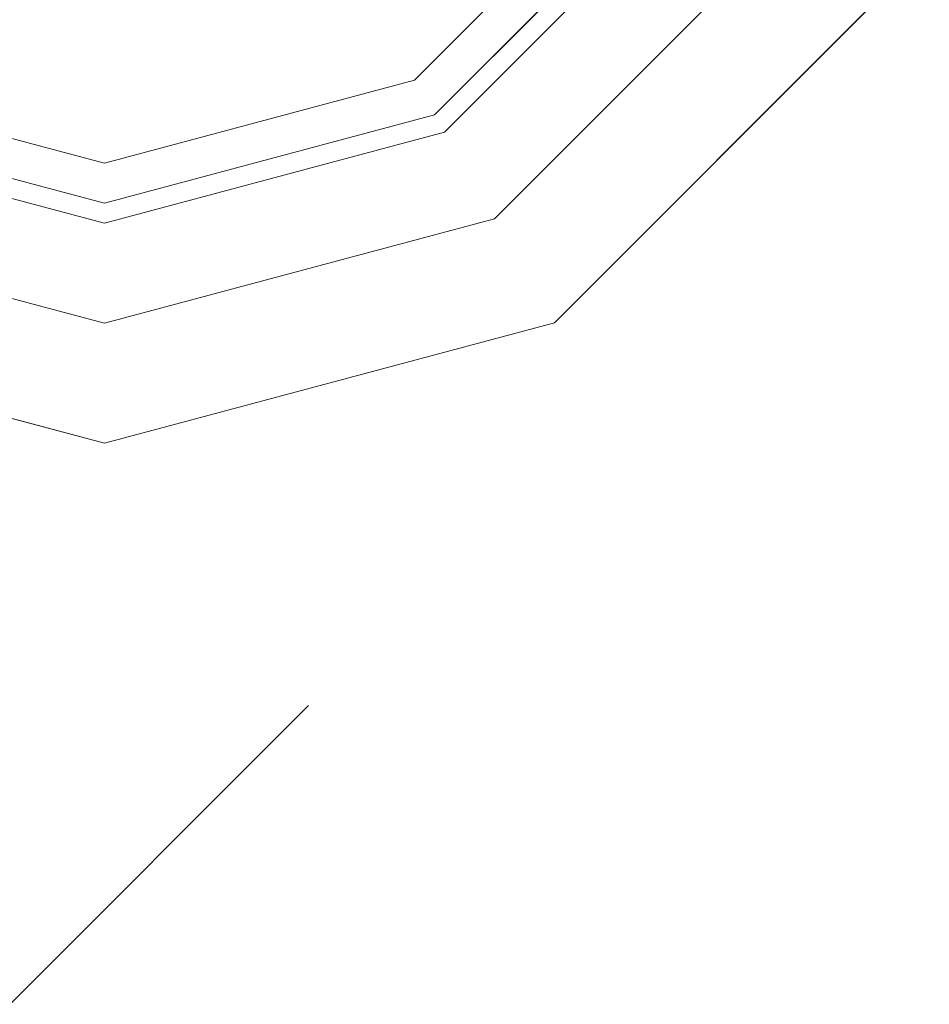
# Model space of a CAD drawing. Units: inches. Extents: x 375 to 1122, y 27 to 1069.
# Tile 134 of 155: x 725.559 to 731.16, y 900.211 to 906.27. Entities that reach past the tile are written whole.
import ezdxf

# ---------------------------------------------------------------- set-up
doc = ezdxf.new("R2010")
doc.units = ezdxf.units.IN
doc.layers.add('A-ANNO-DIMS', color=2, linetype='Continuous', lineweight=18)
doc.layers.add('Furniture', color=30, linetype='Continuous', lineweight=18)
doc.styles.get("Standard").update_dxf_attribs({"font": 'arial.ttf'})
doc.dimstyles.new('ISO-25', dxfattribs={"dimtxt": 12, "dimasz": 2.5, "dimexe": 1.5, "dimexo": 1.5, "dimtad": 1, "dimdec": 1, "dimlunit": 3, "dimtxsty": 'Standard', "dimblk": 'ARCHTICK', "dimcen": 2.5, "dimadec": 0, "dimazin": 0, "dimtfac": 1, "dimtdec": 1, "dimtmove": 0, "dimatfit": 3, "dimfxl": 1.5, "dimfxlon": 1, "dimarcsym": 0})

# ---------------------------------------------------------------- blocks, each defined once
blk = doc.blocks.new('A$C403C54AD')
blk.add_line((0.90685, 1.05977, -0.0006), (1.01943, 0.94723, -0.0006))
at = {"linetype": 'ByBlock'}
for points, invisible_edges in [([(0.81861, 1.08071, -0.03355), (0.84793, 1.09765, -0.02431), (0.79723, 1.14835, -0.02431), (0.7803, 1.11902, -0.03355)], 5), ([(0.84793, 1.09765, -0.0197), (0.83194, 1.08841, -0.0197), (0.78799, 1.13235, -0.0197), (0.79723, 1.14835, -0.0197)], 5), ([(0.83194, 1.08841, -0.0197), (0.81594, 1.07918, -0.02585), (0.77876, 1.11636, -0.02585), (0.78799, 1.13235, -0.0197)], 5), ([(0.81061, 1.0761, -0.04278), (0.81861, 1.08071, -0.03355), (0.7803, 1.11902, -0.03355), (0.77568, 1.11103, -0.04278)], 1), ([(0.81594, 1.07918, -0.02585), (0.72796, 1.02838, -0.02585), (0.72796, 1.02838, -0.02585), (0.77876, 1.11636, -0.02585)], 5), ([(0.83263, 1.02838, -0.03355), (0.86649, 1.02838, -0.02431), (0.84793, 1.09765, -0.02431), (0.81861, 1.08071, -0.03355)], 5), ([(0.86649, 1.02838, -0.0197), (0.84802, 1.02838, -0.0197), (0.83194, 1.08841, -0.0197), (0.84793, 1.09765, -0.0197)], 5), ([(0.84802, 1.02838, -0.0197), (0.82955, 1.02838, -0.02585), (0.81594, 1.07918, -0.02585), (0.83194, 1.08841, -0.0197)], 5), ([(0.82339, 1.02838, -0.04278), (0.83263, 1.02838, -0.03355), (0.81861, 1.08071, -0.03355), (0.81061, 1.0761, -0.04278)], 5), ([(0.82955, 1.02838, -0.02585), (0.72796, 1.02838, -0.02585), (0.72796, 1.02838, -0.02585), (0.81594, 1.07918, -0.02585)], 5), ([(0.81594, 0.97759, -0.02585), (0.72796, 1.02838, -0.02585), (0.72796, 1.02838, -0.02585), (0.82955, 1.02838, -0.02585)], 5), ([(0.77876, 0.94041, -0.02585), (0.72796, 1.02838, -0.02585), (0.72796, 1.02838, -0.02585), (0.81594, 0.97759, -0.02585)], 5), ([(0.81061, 0.98067, -0.04278), (0.81861, 0.97605, -0.03355), (0.83263, 1.02838, -0.03355), (0.82339, 1.02838, -0.04278)], 5), ([(0.83194, 0.96835, -0.0197), (0.81594, 0.97759, -0.02585), (0.82955, 1.02838, -0.02585), (0.84802, 1.02838, -0.0197)], 5), ([(0.81861, 0.97605, -0.03355), (0.84793, 0.95912, -0.02431), (0.86649, 1.02838, -0.02431), (0.83263, 1.02838, -0.03355)], 5), ([(0.84793, 0.95912, -0.0197), (0.83194, 0.96835, -0.0197), (0.84802, 1.02838, -0.0197), (0.86649, 1.02838, -0.0197)], 5)]:
    blk.add_3dface(points, dxfattribs=dict(at, invisible_edges=invisible_edges))
for points in [[(0.84793, 1.09765, -0.02431), (0.84793, 1.09765, -0.0197), (0.79723, 1.14835, -0.0197), (0.79723, 1.14835, -0.02431)], [(0.86649, 1.02838, -0.02431), (0.86649, 1.02838, -0.0197), (0.84793, 1.09765, -0.0197), (0.84793, 1.09765, -0.02431)], [(0.84793, 0.95912, -0.02431), (0.84793, 0.95912, -0.0197), (0.86649, 1.02838, -0.0197), (0.86649, 1.02838, -0.02431)]]:
    blk.add_3dface(points, dxfattribs=at)
blk = doc.blocks.new('_ArchTick')
at = {"color": 0, "linetype": 'ByBlock', "const_width": 0.15}
blk.add_lwpolyline([(-0.5, -0.5), (0.5, 0.5)], dxfattribs=at)
blk = doc.blocks.new('*D73')
at = {"layer": 'A-ANNO-DIMS', "color": 0, "lineweight": -2, "transparency": 16777216}
for p, q in [((686.7573, 932.4277), (686.7573, 929.4277)), ((770.7573, 932.4277), (770.7573, 929.4277)), ((686.7573, 930.9277), (770.7573, 930.9277)), ((770.7573, 930.9277), (987.6096, 930.9277))]:
    blk.add_line(p, q, dxfattribs=at)
at = {"layer": 'Defpoints', "color": 0, "transparency": 16777216}
for p in [(686.7573, 943.5277), (770.7573, 943.5277), (770.7573, 930.9277)]:
    blk.add_point(p, dxfattribs=at)
at = {"layer": 'A-ANNO-DIMS', "color": 0, "lineweight": -2, "transparency": 16777216, "xscale": 2.5, "yscale": 2.5, "zscale": 2.5, "rotation": 180}
blk.add_blockref('_ArchTick', (686.7573, 930.9277), dxfattribs=at)
at = {"layer": 'A-ANNO-DIMS', "color": 0, "lineweight": -2, "transparency": 16777216, "xscale": 2.5, "yscale": 2.5, "zscale": 2.5}
blk.add_blockref('_ArchTick', (770.7573, 930.9277), dxfattribs=at)
at = {"layer": 'A-ANNO-DIMS', "color": 0, "transparency": 16777216, "insert": (880.4335, 937.7573), "char_height": 12, "attachment_point": 5}
blk.add_mtext('2-PANEL SLIDER 7\'-0" TYP.', dxfattribs=at)
blk = doc.blocks.new('*D88')
at = {"layer": 'A-ANNO-DIMS', "color": 0, "lineweight": -2, "transparency": 16777216}
for p, q in [((731.0073, 1052.5277), (731.0073, 1055.5277)), ((854.0073, 1052.5277), (854.0073, 1055.5277)), ((731.0073, 1054.0277), (854.0073, 1054.0277))]:
    blk.add_line(p, q, dxfattribs=at)
at = {"layer": 'Defpoints', "color": 0, "transparency": 16777216}
for p in [(854.0073, 1054.0277), (731.0073, 502.5277), (854.0073, 502.5277)]:
    blk.add_point(p, dxfattribs=at)
at = {"layer": 'A-ANNO-DIMS', "color": 0, "lineweight": -2, "transparency": 16777216, "xscale": 2.5, "yscale": 2.5, "zscale": 2.5, "rotation": 180}
blk.add_blockref('_ArchTick', (731.0073, 1054.0277), dxfattribs=at)
at = {"layer": 'A-ANNO-DIMS', "color": 0, "lineweight": -2, "transparency": 16777216, "xscale": 2.5, "yscale": 2.5, "zscale": 2.5}
blk.add_blockref('_ArchTick', (854.0073, 1054.0277), dxfattribs=at)
at = {"layer": 'A-ANNO-DIMS', "color": 0, "transparency": 16777216, "insert": (792.5073, 1060.7837), "char_height": 12, "attachment_point": 5}
blk.add_mtext('10\'-3"', dxfattribs=at)
blk = doc.blocks.new('*D91')
at = {"layer": 'A-ANNO-DIMS', "color": 0, "lineweight": -2, "transparency": 16777216}
for p, q in [((728.0073, 1052.5277), (728.0073, 1055.5277)), ((788.0073, 1052.5277), (788.0073, 1055.5277)), ((728.0073, 1054.0277), (788.0073, 1054.0277))]:
    blk.add_line(p, q, dxfattribs=at)
at = {"layer": 'Defpoints', "color": 0, "transparency": 16777216}
for p in [(788.0073, 1054.0277), (728.0073, 774.0277), (788.0073, 774.0277)]:
    blk.add_point(p, dxfattribs=at)
at = {"layer": 'A-ANNO-DIMS', "color": 0, "lineweight": -2, "transparency": 16777216, "xscale": 2.5, "yscale": 2.5, "zscale": 2.5, "rotation": 180}
blk.add_blockref('_ArchTick', (728.0073, 1054.0277), dxfattribs=at)
at = {"layer": 'A-ANNO-DIMS', "color": 0, "lineweight": -2, "transparency": 16777216, "xscale": 2.5, "yscale": 2.5, "zscale": 2.5}
blk.add_blockref('_ArchTick', (788.0073, 1054.0277), dxfattribs=at)
at = {"layer": 'A-ANNO-DIMS', "color": 0, "transparency": 16777216, "insert": (758.0073, 1060.7796), "char_height": 12, "attachment_point": 5}
blk.add_mtext('5\'-0"', dxfattribs=at)

msp = doc.modelspace()

# ---------------------------------------------------------------- block references
at = {"layer": 'Furniture', "xscale": 39.9918517141215, "yscale": 39.9918517141215, "zscale": 39.9918517141215, "rotation": 270}
msp.add_blockref('A$C403C54AD', (684.9549, 938.3156, 0.024), dxfattribs=at)

# ---------------------------------------------------------------- dimensions: what is measured, and where the dimension line sits
at = {"layer": 'A-ANNO-DIMS'}
for base, p1, p2, picture, middle in [((788.0073, 1054.0277), (728.0073, 774.0277), (788.0073, 774.0277), '*D91', (758.0073, 1060.7796)), ((854.0073, 1054.0277), (731.0073, 502.5277), (854.0073, 502.5277), '*D88', (792.5073, 1060.7837))]:
    dim = msp.add_linear_dim(base=base, p1=p1, p2=p2, dimstyle='ISO-25', override={"dimdec": 1, "dimlfac": 1, "dimrnd": 0, "dimzin": 1, "dimdsep": 46, "dimlunit": 4, "dimfrac": 2}, dxfattribs=at)
    dim.commit()
    dim.dimension.update_dxf_attribs({"geometry": picture, "text_midpoint": middle})
dim = msp.add_linear_dim(base=(770.7573, 930.9277), p1=(686.7573, 943.5277), p2=(770.7573, 943.5277), text='2-PANEL SLIDER <> TYP.', dimstyle='ISO-25', override={"dimdec": 1, "dimlfac": 1, "dimrnd": 0, "dimzin": 1, "dimdsep": 46, "dimlunit": 4, "dimfrac": 2}, dxfattribs=at)
dim.commit()
dim.dimension.update_dxf_attribs({"geometry": '*D73', "text_midpoint": (880.4335, 937.7573)})

doc.saveas('drawing.dxf')
